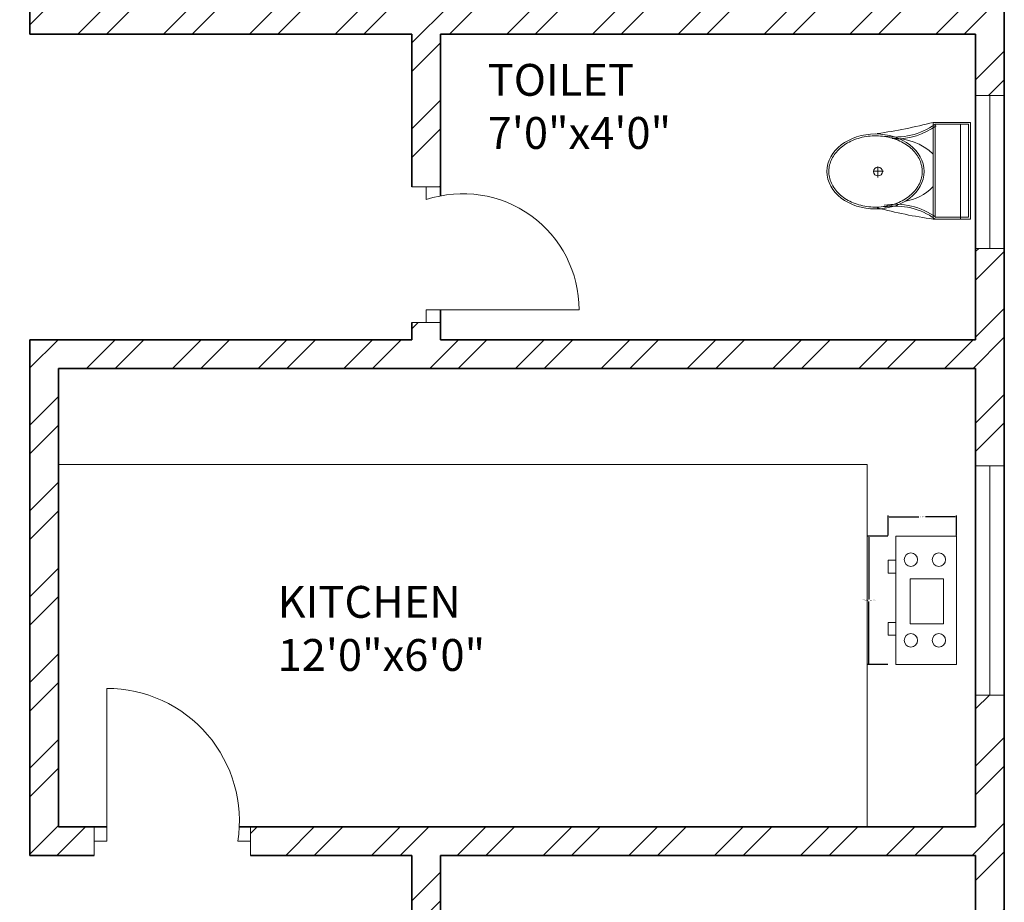
# Model space of a CAD drawing. Units: inches. Extents: x 1962 to 2771, y 1245 to 2660.
# Tile 20 of 114: x 2506 to 2661, y 1692 to 1831. Entities that reach past the tile are written whole.
import ezdxf

# ---------------------------------------------------------------- set-up
doc = ezdxf.new("R2010")
doc.units = ezdxf.units.IN
for name, color, linetype, lineweight in [('A-ANNO-DIMS', 2, 'Continuous', 18), ('A-AREA-IDEN', 7, 'Continuous', 18), ('A-DOOR', 3, 'Continuous', 18), ('A-EQPM', 8, 'Continuous', 18), ('A-FLOR-CASE', 8, 'Continuous', 18), ('A-FLOR-FIXT', 8, 'Continuous', 18), ('A-GLAZ', 4, 'Continuous', 18), ('A-WALL', 7, 'Continuous', 35), ('A-WALL-PATT', 252, 'Continuous', 13)]:
    doc.layers.add(name, color=color, linetype=linetype, lineweight=lineweight)
doc.styles.get("Standard").update_dxf_attribs({"font": 'arial.ttf'})
doc.dimstyles.get("Standard").update_dxf_attribs({"dimtxt": 0.18, "dimasz": 0.18, "dimexe": 0.18, "dimexo": 0.0625, "dimgap": 0.09, "dimtad": 0, "dimtih": 1, "dimtoh": 1, "dimdec": 4, "dimzin": 0, "dimdsep": 46, "dimtxsty": 'Standard', "dimcen": 0.09, "dimadec": 0, "dimazin": 0, "dimtfac": 1, "dimtdec": 4, "dimtofl": 0, "dimtmove": 0, "dimatfit": 3, "dimfxl": 1, "dimtolj": 1, "dimtzin": 0, "dimarcsym": 0})

# ---------------------------------------------------------------- blocks, each defined once
blk = doc.blocks.new('A$C31115884')
for p, q in [((283.1, 497.7), (223.4, 497.7)), ((257.5, 466.4), (257.5, 523.2)), ((0, 200), (0, 0)), ((520, 200), (0, 200)), ((10, 190), (10, 10)), ((510, 190), (10, 190)), ((510, 10), (510, 190)), ((520, 0), (520, 200)), ((510, 54.5), (0, 54.5)), ((10, 10), (510, 10)), ((0, 0), (520, 0))]:
    blk.add_line(p, q)
blk.add_circle((255.6, 496.4), 23.6)
for centre, radius, start, end in [((2777.7, -204.6), 2807, 165.4549, 171.7133), ((3237, 905), 2807, 188.2867, 194.5451), ((-294.5, 403.3), 364.7, 324.2091, 9.3499), ((-294.5, 403.3), 374.7, 324.2091, 9.3499), ((805.8, 403.3), 364.7, 170.6501, 215.7909), ((139.5, 406.2), 293.5, 315.8436, 2.6563), ((805.8, 403.3), 374.7, 179.2036, 215.7909), ((383.6, 406.2), 293.5, 190.2774, 224.1564)]:
    blk.add_arc(centre, radius, start, end)
blk.add_ellipse((256.2, 509.9), major_axis=(0, -260.7), ratio=0.772727)
blk.add_open_spline([(256.2, 259.2), (263.1, 259.2), (270, 259.7), (287.8, 262.3), (298.7, 265.1), (319.9, 273.1), (330.2, 278.4), (350.1, 291.1), (359.7, 298.7), (377.7, 315.9), (386.2, 325.5), (401.7, 346.6), (408.8, 358.1), (421.3, 382.5), (426.8, 395.5), (435.9, 422.4), (439.5, 436.4), (444.8, 465.1), (446.5, 479.7), (447.9, 509.2), (447.6, 524), (445, 553.3), (442.7, 567.8), (436.3, 596), (432.1, 609.7), (421.9, 636), (416, 648.6), (402.5, 672.1), (395, 683), (378.6, 703), (369.8, 712.1), (351.1, 728), (341.3, 734.8), (320.9, 746.2), (310.4, 750.7), (288.9, 757.3), (278, 759.4), (256, 761), (245, 760.6), (223.1, 757.2), (212.3, 754.3), (191.1, 746.1), (180.8, 740.7), (160.9, 727.8), (151.4, 720.1), (133.5, 702.7), (125.1, 693), (109.6, 671.7), (102.6, 660.2), (90.2, 635.7), (84.9, 622.7), (76, 595.6), (72.4, 581.6), (67.2, 552.9), (65.6, 538.2), (64.4, 508.8), (64.8, 494), (67.5, 464.7), (69.9, 450.2), (76.6, 422), (80.8, 408.3), (91.1, 382.2), (97.2, 369.7), (110.8, 346.3), (118.4, 335.4), (134.8, 315.6), (143.7, 306.7), (162.4, 290.9), (172.3, 284.2), (192.8, 273), (203.3, 268.6), (224.8, 262.2), (235.8, 260.2), (249.9, 259.3), (253, 259.2), (256.2, 259.2)], degree=3, knots=[0, 0, 0, 0, 0.110105, 0.110105, 0.285049, 0.285049, 0.459994, 0.459994, 0.634938, 0.634938, 0.809882, 0.809882, 0.984827, 0.984827, 1.159771, 1.159771, 1.334715, 1.334715, 1.50966, 1.50966, 1.684604, 1.684604, 1.859549, 1.859549, 2.034493, 2.034493, 2.209437, 2.209437, 2.384382, 2.384382, 2.559326, 2.559326, 2.73427, 2.73427, 2.909215, 2.909215, 3.084159, 3.084159, 3.259103, 3.259103, 3.434048, 3.434048, 3.608992, 3.608992, 3.783936, 3.783936, 3.958881, 3.958881, 4.133825, 4.133825, 4.30877, 4.30877, 4.483714, 4.483714, 4.658658, 4.658658, 4.833603, 4.833603, 5.008547, 5.008547, 5.183491, 5.183491, 5.358436, 5.358436, 5.53338, 5.53338, 5.708324, 5.708324, 5.883269, 5.883269, 6.058213, 6.058213, 6.233158, 6.233158, 6.283185, 6.283185, 6.283185, 6.283185])
blk = doc.blocks.new('COOKTOP-4-BURNER')
for points in [[(0, 20.18), (9.48, 20.18), (9.48, 0), (0, 0)], [(9.48, 15.59), (10.71, 15.59), (10.71, 13.59), (9.48, 13.59)], [(2, 13.79), (7.26, 13.79), (7.26, 6.73), (2, 6.73)], [(9.48, 5.81), (10.71, 5.81), (10.71, 3.8), (9.48, 3.8)]]:
    blk.add_lwpolyline(points, close=True)
for centre in [(2.74, 16.38), (7.14, 16.38), (2.74, 3.71), (7.14, 3.71)]:
    blk.add_circle(centre, 1.05)
blk = doc.blocks.new('WIN-24IN-A')
for p, q in [((0, 24), (4.5, 24)), ((4.5, 24), (2.25, 24)), ((2.25, 24), (2.25, 0)), ((2.25, 0), (0, 0)), ((0, 0), (4.5, 0))]:
    blk.add_line(p, q)
blk = doc.blocks.new('WIN-36IN-B')
for p, q in [((0, 36), (4.5, 36)), ((4.5, 36), (2.25, 36)), ((2.25, 36), (2.25, 0)), ((2.25, 0), (0, 0)), ((0, 0), (4.5, 0))]:
    blk.add_line(p, q)
blk = doc.blocks.new('*D30')
at = {"layer": 'A-ANNO-DIMS', "color": 0, "lineweight": -2, "transparency": 16777216}
for p, q in [((2642.51, 1749.52), (2639.37, 1749.52)), ((2639.55, 1749.34), (2639.55, 1739.61)), ((2639.55, 1729.52), (2639.55, 1739.25)), ((2642.51, 1729.34), (2639.37, 1729.34))]:
    blk.add_line(p, q, dxfattribs=at)
at = {"layer": 'A-ANNO-DIMS', "color": 0, "transparency": 16777216}
for points in [[(2639.52, 1749.34), (2639.58, 1749.34), (2639.55, 1749.52)], [(2639.52, 1729.52), (2639.58, 1729.52), (2639.55, 1729.34)]]:
    blk.add_solid(points, dxfattribs=at)
at = {"layer": 'Defpoints', "color": 0, "transparency": 16777216}
for p in [(2642.57, 1749.52), (2639.55, 1729.34), (2642.57, 1729.34)]:
    blk.add_point(p, dxfattribs=at)
at = {"layer": 'A-ANNO-DIMS', "color": 0, "transparency": 16777216, "insert": (2639.55, 1739.43), "char_height": 0.18, "attachment_point": 5}
blk.add_mtext('\\A1;COOKTOP 20 TYP.', dxfattribs=at)
blk = doc.blocks.new('*D31')
at = {"layer": 'A-ANNO-DIMS', "color": 0, "lineweight": -2, "transparency": 16777216}
for p, q in [((2642.57, 1749.58), (2642.57, 1752.72)), ((2642.75, 1752.54), (2647.41, 1752.54)), ((2653.1, 1752.54), (2648.45, 1752.54)), ((2653.28, 1749.58), (2653.28, 1752.72))]:
    blk.add_line(p, q, dxfattribs=at)
at = {"layer": 'A-ANNO-DIMS', "color": 0, "transparency": 16777216}
for points in [[(2642.75, 1752.57), (2642.75, 1752.51), (2642.57, 1752.54)], [(2653.1, 1752.57), (2653.1, 1752.51), (2653.28, 1752.54)]]:
    blk.add_solid(points, dxfattribs=at)
at = {"layer": 'Defpoints', "color": 0, "transparency": 16777216}
for p in [(2642.57, 1752.54), (2642.57, 1749.52), (2653.28, 1749.52)]:
    blk.add_point(p, dxfattribs=at)
at = {"layer": 'A-ANNO-DIMS', "color": 0, "transparency": 16777216, "insert": (2647.93, 1752.54), "char_height": 0.18, "attachment_point": 5}
blk.add_mtext('\\A1;11 TYP.', dxfattribs=at)

msp = doc.modelspace()

# ---------------------------------------------------------------- hatches: boundary and pattern name
at = {"layer": 'A-WALL-PATT'}
h = msp.add_hatch(dxfattribs=at)
h.set_pattern_fill('ANSI32', color=256)
h.paths.add_polyline_path([(2090.8074, 2467.3437), (2141.6481, 2467.3437), (2141.6481, 2469.5937), (2141.6481, 2471.8437), (2086.3074, 2471.8437), (2086.3074, 2422.5333), (2090.8074, 2422.5333)])
h.paths.add_polyline_path([(2282.7664, 2471.8437), (2204.8982, 2471.8437), (2204.8982, 2467.3437), (2234.8074, 2467.3437), (2234.8074, 2311.3437), (2228.7492, 2311.3437), (2228.7492, 2306.8437), (2234.8074, 2306.8437), (2331.9227, 2306.8437), (2331.9227, 2309.0937), (2331.9227, 2311.3437), (2239.3074, 2311.3437), (2239.3074, 2467.3437), (2282.7664, 2467.3437), (2282.7664, 2469.5937)])
h.paths.add_polyline_path([(2471.4531, 2519.8437), (2552.011, 2519.8437), (2564.3996, 2519.8437), (2564.3996, 2511.1389), (2568.8996, 2511.1389), (2568.8996, 2524.3437), (2466.9531, 2524.3437), (2466.9531, 2471.8437), (2450.0749, 2471.8437), (2446.4672, 2471.8437), (2446.4672, 2467.3437), (2450.0749, 2467.3437), (2475.9988, 2467.3437), (2475.9988, 2469.5937), (2475.9988, 2471.8437), (2471.4531, 2471.8437)])
h.paths.add_polyline_path([(2575.2231, 2469.5937), (2575.2231, 2471.8437), (2568.8996, 2471.8437), (2568.8996, 2487.1389), (2564.3996, 2487.1389), (2564.3996, 2471.8437), (2556.511, 2471.8437), (2499.2904, 2471.8437), (2499.2904, 2467.3437), (2507.8074, 2467.3437), (2507.8074, 2311.3437), (2414.863, 2311.3437), (2414.863, 2306.8437), (2512.3074, 2306.8437), (2517.0114, 2306.8437), (2517.0114, 2309.0937), (2517.0114, 2311.3437), (2512.3074, 2311.3437), (2512.3074, 2467.3437), (2575.2231, 2467.3437)])
h.paths.add_polyline_path([(2660.8074, 2471.8437), (2600.9602, 2471.8437), (2600.9602, 2467.3437), (2656.3074, 2467.3437), (2656.3074, 2432.5704), (2660.8074, 2432.5704)])
h.paths.add_polyline_path([(2660.8074, 2372.5704), (2656.3074, 2372.5704), (2656.3074, 2311.3437), (2600.276, 2311.3437), (2600.276, 2309.0937), (2600.276, 2306.8437), (2656.3074, 2306.8437), (2656.3074, 2296.2593), (2660.8074, 2296.2593)])
h.paths.add_polyline_path([(2572.3074, 2306.8437), (2577.1385, 2306.8437), (2577.1385, 2311.3437), (2551.082, 2311.3437), (2551.082, 2306.8437), (2567.8074, 2306.8437), (2567.8074, 2258.8437), (2540.0574, 2258.8437), (2540.0574, 2256.5937), (2540.0574, 2254.3437), (2567.8074, 2254.3437), (2656.3074, 2254.3437), (2656.3074, 2236.9085), (2660.8074, 2236.9085), (2660.8074, 2272.2593), (2656.3074, 2272.2593), (2656.3074, 2258.8437), (2572.3074, 2258.8437)])
h.paths.add_polyline_path([(2512.3074, 2254.3437), (2518.8716, 2254.3437), (2518.8716, 2256.5937), (2518.8716, 2258.8437), (2507.8074, 2258.8437), (2507.8074, 2177.8437), (2567.8074, 2177.8437), (2567.8074, 2172.9628), (2572.3074, 2172.9628), (2572.3074, 2177.8437), (2656.3074, 2177.8437), (2656.3074, 2166.4846), (2660.8074, 2166.4846), (2660.8074, 2200.9085), (2656.3074, 2200.9085), (2656.3074, 2182.3437), (2512.3074, 2182.3437)])
h.paths.add_polyline_path([(2656.3074, 2129.8437), (2572.3074, 2129.8437), (2572.3074, 2150.3044), (2570.0574, 2150.3044), (2567.8074, 2150.3044), (2567.8074, 2129.8437), (2507.8074, 2129.8437), (2507.8074, 2116.3027), (2510.0574, 2116.3027), (2512.3074, 2116.3027), (2512.3074, 2125.3437), (2567.8074, 2125.3437), (2572.3074, 2125.3437), (2656.3074, 2125.3437)])
h.paths.add_polyline_path([(2090.8074, 2362.5333), (2086.3074, 2362.5333), (2086.3074, 2298.6242), (2090.8074, 2298.6242), (2090.8074, 2306.8437), (2174.8074, 2306.8437), (2174.8074, 2286.4178), (2179.3074, 2286.4178), (2179.3074, 2306.8437), (2192.8641, 2306.8437), (2192.8641, 2309.0937), (2192.8641, 2311.3437), (2090.8074, 2311.3437)])
h.paths.add_polyline_path([(2209.156, 2258.8437), (2179.3074, 2258.8437), (2179.3074, 2263.2236), (2177.0574, 2263.2236), (2174.8074, 2263.2236), (2174.8074, 2258.8437), (2090.8074, 2258.8437), (2090.8074, 2274.6242), (2086.3074, 2274.6242), (2086.3074, 2238.2967), (2088.5574, 2238.2967), (2090.8074, 2238.2967), (2090.8074, 2254.3437), (2209.156, 2254.3437)])
h.paths.add_polyline_path([(2090.8074, 2177.8437), (2234.8074, 2177.8437), (2234.8074, 2173.1428), (2239.3074, 2173.1428), (2239.3074, 2258.8437), (2230.8442, 2258.8437), (2230.8442, 2256.5937), (2230.8442, 2254.3437), (2234.8074, 2254.3437), (2234.8074, 2182.3437), (2090.8074, 2182.3437), (2090.8074, 2202.2967), (2086.3074, 2202.2967), (2086.3074, 2140.0389), (2090.8074, 2140.0389)])
h.paths.add_polyline_path([(2090.8074, 2080.0389), (2086.3074, 2080.0389), (2086.3074, 2033.8437), (2090.8074, 2033.8437)], flags=17)
h.paths.add_polyline_path([(2244.9405, 2033.8437), (2239.3074, 2033.8437), (2239.3074, 2142.0665), (2237.2592, 2142.0665), (2234.8074, 2142.0665), (2234.8074, 2033.8437), (2090.8074, 2033.8437), (2076.5204, 2033.8437), (2072.0204, 2033.8437), (2072.0204, 2000.4493), (2076.5204, 2000.4493), (2076.5204, 2029.3437), (2090.8074, 2029.3437), (2244.9405, 2029.3437), (2244.9405, 2031.5937)])
h.paths.add_polyline_path([(2234.8074, 1933.3437), (2076.5204, 1933.3437), (2076.5204, 1952.4493), (2074.2704, 1952.4493), (2072.0204, 1952.4493), (2072.0204, 1933.3437), (2072.0204, 1928.8437), (2234.8074, 1928.8437)])
h.paths.add_polyline_path([(2090.8074, 1928.8437), (2086.3074, 1928.8437), (2086.3074, 1906.5013), (2090.8074, 1906.5013)])
h.paths.add_polyline_path([(2090.8074, 1846.5013), (2086.3074, 1846.5013), (2086.3074, 1769.9917), (2088.5574, 1769.9917), (2090.8074, 1769.9917), (2090.8074, 1780.3437), (2234.8074, 1780.3437), (2234.8074, 1708.3437), (2230.3764, 1708.3437), (2230.3764, 1703.8437), (2239.3074, 1703.8437), (2239.3074, 1792.6669), (2237.0574, 1792.6669), (2234.8074, 1792.6669), (2234.8074, 1784.8437), (2090.8074, 1784.8437)])
h.paths.add_polyline_path([(2239.3074, 1928.8437), (2244.9405, 1928.8437), (2244.9405, 1931.0937), (2244.9405, 1933.3437), (2234.8074, 1933.3437), (2234.8074, 1928.8437), (2234.8074, 1825.5949), (2239.3074, 1825.5949)])
h.paths.add_polyline_path([(2148.0425, 1649.0937), (2148.0425, 1651.3437), (2090.8074, 1651.3437), (2090.8074, 1646.8437), (2148.0425, 1646.8437)], flags=0)
h.paths.add_polyline_path([(2207.5601, 1708.3437), (2090.8074, 1708.3437), (2090.8074, 1703.8437), (2174.8074, 1703.8437), (2174.8074, 1651.3437), (2170.4457, 1651.3437), (2170.4457, 1646.8437), (2195.9924, 1646.8437), (2195.9924, 1649.0937), (2195.9924, 1651.3437), (2179.3074, 1651.3437), (2179.3074, 1703.8437), (2207.5601, 1703.8437), (2207.5601, 1706.0937)])
h.paths.add_polyline_path([(2090.8074, 1733.9917), (2086.3074, 1733.9917), (2086.3074, 1696.1032), (2088.5574, 1696.1032), (2090.8074, 1696.1032)])
h.paths.add_polyline_path([(2090.8074, 1672.1032), (2086.3074, 1672.1032), (2086.3074, 1600.3335), (2090.8074, 1600.3335)])
h.paths.add_polyline_path([(2090.8074, 1540.3335), (2086.3074, 1540.3335), (2086.3074, 1486.3437), (2139.6766, 1486.3437), (2139.6766, 1490.8437), (2090.8074, 1490.8437)])
h.paths.add_polyline_path([(2302.3876, 1490.8437), (2239.3074, 1490.8437), (2239.3074, 1646.8437), (2335.9994, 1646.8437), (2335.9994, 1651.3437), (2229.884, 1651.3437), (2229.884, 1646.8437), (2234.8074, 1646.8437), (2234.8074, 1490.8437), (2202.7103, 1490.8437), (2202.7103, 1488.5937), (2202.7103, 1486.3437), (2275.0699, 1486.3437), (2275.0699, 1475.772), (2279.5699, 1475.772), (2279.5699, 1486.3437), (2302.3876, 1486.3437)])
h.paths.add_polyline_path([(2279.5699, 1451.772), (2275.0699, 1451.772), (2275.0699, 1438.3437), (2174.8074, 1438.3437), (2174.8074, 1486.3437), (2179.7922, 1486.3437), (2179.7922, 1490.8437), (2163.3585, 1490.8437), (2163.3585, 1488.5937), (2163.3585, 1486.3437), (2170.3074, 1486.3437), (2170.3074, 1433.8437), (2279.5699, 1433.8437)])
h.paths.add_polyline_path([(2427.2363, 1490.8437), (2375.8074, 1490.8437), (2375.8074, 1646.8437), (2381.6401, 1646.8437), (2381.6401, 1651.3437), (2365.887, 1651.3437), (2365.887, 1649.0937), (2365.887, 1646.8437), (2371.3074, 1646.8437), (2371.3074, 1490.8437), (2327.5627, 1490.8437), (2327.5627, 1488.5937), (2327.5627, 1486.3437), (2371.3074, 1486.3437), (2371.3074, 1433.8437), (2375.8074, 1433.8437), (2375.8074, 1486.3437), (2427.2363, 1486.3437)])
h.paths.add_polyline_path([(2512.3074, 1646.8437), (2519.4351, 1646.8437), (2519.4351, 1649.0937), (2519.4351, 1651.3437), (2507.8074, 1651.3437), (2416.0063, 1651.3437), (2416.0063, 1649.0937), (2416.0063, 1646.8437), (2507.8074, 1646.8437), (2507.8074, 1490.8437), (2497.0532, 1490.8437), (2497.0532, 1488.5937), (2497.0532, 1486.3437), (2574.9344, 1486.3437), (2574.9344, 1476.0181), (2579.4344, 1476.0181), (2579.4344, 1486.3437), (2584.4872, 1486.3437), (2584.3074, 1490.8437), (2512.3074, 1490.8437)])
h.paths.add_polyline_path([(2470.5091, 1486.3437), (2473.9767, 1486.3437), (2473.9767, 1490.8437), (2449.6605, 1490.8437), (2449.6605, 1488.5937), (2449.6605, 1486.3437), (2466.0091, 1486.3437), (2466.0091, 1433.8437), (2470.5091, 1433.8437), (2579.4344, 1433.8437), (2579.4344, 1452.0181), (2574.9344, 1452.0181), (2574.9344, 1438.3437), (2554.5091, 1438.3437), (2470.5091, 1438.3437)])
h.paths.add_polyline_path([(2656.3074, 1490.8437), (2611.86, 1490.8437), (2611.86, 1486.3437), (2656.3074, 1486.3437)])
h.paths.add_polyline_path([(2660.8074, 1532.7007), (2658.5574, 1532.7007), (2656.3074, 1532.7007), (2656.3074, 1486.3437), (2660.8074, 1486.3437)])
h.paths.add_polyline_path([(2660.8074, 1664.9663), (2656.3074, 1664.9663), (2656.3074, 1651.3437), (2602.2313, 1651.3437), (2602.2313, 1646.8437), (2656.3074, 1646.8437), (2656.3074, 1592.7007), (2660.8074, 1592.7007)])
h.paths.add_polyline_path([(2660.8074, 1724.5221), (2656.3074, 1724.5221), (2656.3074, 1703.8437), (2542.4725, 1703.8437), (2542.4725, 1699.3437), (2567.8074, 1699.3437), (2567.8074, 1651.3437), (2552.7766, 1651.3437), (2552.7766, 1649.0937), (2552.7766, 1646.8437), (2577.2878, 1646.8437), (2577.2878, 1649.0937), (2577.2878, 1651.3437), (2572.3074, 1651.3437), (2572.3074, 1699.3437), (2656.3074, 1699.3437), (2656.3074, 1688.9663), (2660.8074, 1688.9663)])
h.paths.add_polyline_path([(2660.8074, 1880.6524), (2656.3074, 1880.6524), (2656.3074, 1832.8437), (2512.3074, 1832.8437), (2512.3074, 1837.8959), (2507.8074, 1837.8959), (2507.8074, 1828.3437), (2567.8074, 1828.3437), (2567.8074, 1804.3437), (2572.3074, 1804.3437), (2572.3074, 1828.3437), (2656.3074, 1828.3437), (2656.3074, 1818.6778), (2660.8074, 1818.6778)])
h.paths.add_polyline_path([(2660.8074, 1794.6778), (2656.3074, 1794.6778), (2656.3074, 1780.3437), (2572.3074, 1780.3437), (2572.3074, 1783.0303), (2570.0574, 1783.0303), (2567.8074, 1783.0303), (2567.8074, 1780.3437), (2507.8074, 1780.3437), (2507.8074, 1699.3437), (2517.8858, 1699.3437), (2517.8858, 1701.5937), (2517.8858, 1703.8437), (2512.3074, 1703.8437), (2512.3074, 1775.8437), (2656.3074, 1775.8437), (2656.3074, 1760.5221), (2660.8074, 1760.5221)])
h.paths.add_polyline_path([(2660.8074, 1981.3437), (2660.8074, 2020.2808), (2658.5574, 2020.2808), (2656.3074, 2020.2808), (2656.3074, 1981.3437), (2512.3074, 1981.3437), (2512.3074, 2086.6996), (2507.8074, 2086.6996), (2507.8074, 1981.3437), (2375.8074, 1981.3437), (2375.8074, 1986.8505), (2373.5574, 1986.8505), (2371.3074, 1986.8505), (2371.3074, 1973.2607), (2375.8074, 1973.2607), (2375.8074, 1976.8437), (2507.8074, 1976.8437), (2507.8074, 1865.4281), (2510.0574, 1865.4281), (2512.3074, 1865.4281), (2512.3074, 1976.8437), (2660.8074, 1976.8437)])
h.paths.add_polyline_path([(2375.8074, 1940.297), (2373.5574, 1940.297), (2371.3074, 1940.297), (2371.3074, 1933.3437), (2278.4434, 1933.3437), (2278.4434, 1928.8437), (2371.3074, 1928.8437), (2371.3074, 1651.3437), (2375.8074, 1651.3437)])
h.paths.add_polyline_path([(2660.8074, 1976.8437), (2656.3074, 1976.8437), (2656.3074, 1940.6524), (2660.8074, 1940.6524)], flags=17)
h.paths.add_polyline_path([(2660.8074, 2142.4846), (2656.3074, 2142.4846), (2656.3074, 2080.2808), (2660.8074, 2080.2808)])
h.paths.add_polyline_path([(2381.4189, 2311.3437), (2375.8074, 2311.3437), (2375.8074, 2467.3437), (2424.7242, 2467.3437), (2424.7242, 2469.5937), (2424.7242, 2471.8437), (2375.8074, 2471.8437), (2375.8074, 2524.3437), (2371.3074, 2524.3437), (2371.3074, 2471.8437), (2307.2097, 2471.8437), (2307.2097, 2467.3437), (2371.3074, 2467.3437), (2371.3074, 2311.3437), (2366.8901, 2311.3437), (2366.8901, 2306.8437), (2371.3074, 2306.8437), (2371.3074, 2033.8437), (2279.6589, 2033.8437), (2279.6589, 2029.3437), (2371.3074, 2029.3437), (2371.3074, 2014.2598), (2375.8074, 2014.2598), (2375.8074, 2306.8437), (2381.4189, 2306.8437)])
h.paths.add_polyline_path([(2263.3074, 2524.3437), (2170.3074, 2524.3437), (2170.3074, 2519.8437), (2170.3074, 2471.8437), (2165.0312, 2471.8437), (2165.0312, 2467.3437), (2179.6721, 2467.3437), (2179.6721, 2469.5161), (2179.6721, 2471.8437), (2174.8074, 2471.8437), (2174.8074, 2519.8437), (2258.8074, 2519.8437), (2258.8074, 2511.6436), (2263.3074, 2511.6436)])
h.paths.add_polyline_path([(2245.0232, 1361.4123), (2492.9468, 1361.4123), (2492.9468, 1398.505), (2245.0232, 1398.505)], flags=9)
h.paths.add_polyline_path([(2388.1434, 2086.6936), (2425.0704, 2086.6936), (2425.0704, 2105.3509), (2388.1434, 2105.3509)], flags=9)
h.paths.add_polyline_path([(2404.922, 2242.6744), (2445.7337, 2242.6744), (2445.7337, 2261.3318), (2404.922, 2261.3318)], flags=9)
h.paths.add_polyline_path([(2269.4107, 2156.7935), (2306.3378, 2156.7935), (2306.3378, 2175.4508), (2269.4107, 2175.4508)], flags=9)
h.paths.add_polyline_path([(2269.3277, 2233.4343), (2306.2547, 2233.4343), (2306.2547, 2252.0917), (2269.3277, 2252.0917)], flags=9)
h.paths.add_polyline_path([(2431.6052, 2320.6922), (2470.4456, 2320.6922), (2470.4456, 2339.3495), (2431.6052, 2339.3495)], flags=25)
h.paths.add_polyline_path([(2249.6902, 2315.7608), (2288.5306, 2315.7608), (2288.5306, 2334.4182), (2249.6902, 2334.4182)], flags=25)
h.paths.add_polyline_path([(2096.9301, 2314.3181), (2135.7704, 2314.3181), (2135.7704, 2332.9755), (2096.9301, 2332.9755)], flags=25)
h.paths.add_polyline_path([(2134.3475, 2285.7089), (2161.4655, 2285.7089), (2161.4655, 2304.3662), (2134.3475, 2304.3662)], flags=9)
h.paths.add_polyline_path([(2126.5155, 2209.4076), (2159.9227, 2209.4076), (2159.9227, 2228.065), (2126.5155, 2228.065)], flags=25)
h.paths.add_polyline_path([(2110.5753, 2141.5299), (2149.4157, 2141.5299), (2149.4157, 2160.1872), (2110.5753, 2160.1872)], flags=25)
h.paths.add_polyline_path([(2249.8618, 1968.3317), (2286.3966, 1968.3317), (2286.3966, 1986.989), (2249.8618, 1986.989)], flags=9)
h.paths.add_polyline_path([(2395.9507, 1777.0051), (2436.7624, 1777.0051), (2436.7624, 1795.6625), (2395.9507, 1795.6625)], flags=9)
h.paths.add_polyline_path([(2398.5259, 1888.5651), (2435.0062, 1888.5651), (2435.0062, 1907.2224), (2398.5259, 1907.2224)], flags=25)
h.paths.add_polyline_path([(2259.3506, 1728.3559), (2296.2776, 1728.3559), (2296.2776, 1747.0132), (2259.3506, 1747.0132)], flags=9)
h.paths.add_polyline_path([(2271.3698, 1845.268), (2308.2968, 1845.268), (2308.2968, 1863.9253), (2271.3698, 1863.9253)], flags=9)
h.paths.add_polyline_path([(2120.9355, 1786.3027), (2159.7759, 1786.3027), (2159.7759, 1804.9601), (2120.9355, 1804.9601)], flags=25)
h.paths.add_polyline_path([(2121.3164, 1732.1043), (2154.7236, 1732.1043), (2154.7236, 1750.7616), (2121.3164, 1750.7616)], flags=25)
h.paths.add_polyline_path([(2118.3706, 1678.8997), (2147.5282, 1678.8997), (2147.5282, 1697.557), (2118.3706, 1697.557)], flags=25)
h.paths.add_polyline_path([(2385.9227, 1493.557), (2424.763, 1493.557), (2424.763, 1512.2143), (2385.9227, 1512.2143)], flags=25)
h.paths.add_polyline_path([(2248.7058, 1500.0256), (2287.5462, 1500.0256), (2287.5462, 1518.6829), (2248.7058, 1518.6829)], flags=25)
h.paths.add_polyline_path([(2104.1669, 1617.3771), (2143.0073, 1617.3771), (2143.0073, 1636.0344), (2104.1669, 1636.0344)], flags=9)
h.paths.add_polyline_path([(2096.0714, 1447.8824), (2137.3845, 1447.8824), (2137.3845, 1458.1859), (2096.0714, 1458.1859)], flags=9)
h.paths.add_polyline_path([(2180.6114, 1440.325), (2209.7689, 1440.325), (2209.7689, 1458.9823), (2180.6114, 1458.9823)], flags=25)
h.paths.add_polyline_path([(2316.1698, 1447.9637), (2357.4829, 1447.9637), (2357.4829, 1458.2673), (2316.1698, 1458.2673)], flags=9)
h.paths.add_polyline_path([(2397.6187, 1447.9637), (2438.9318, 1447.9637), (2438.9318, 1458.2673), (2397.6187, 1458.2673)], flags=9)
h.paths.add_polyline_path([(2473.0778, 1439.5953), (2502.2354, 1439.5953), (2502.2354, 1458.2527), (2473.0778, 1458.2527)], flags=25)
h.paths.add_polyline_path([(2589.7027, 1447.8819), (2631.0158, 1447.8819), (2631.0158, 1458.1855), (2589.7027, 1458.1855)], flags=9)
h.paths.add_polyline_path([(2522.4009, 1497.5285), (2561.2413, 1497.5285), (2561.2413, 1516.1859), (2522.4009, 1516.1859)], flags=25)
h.paths.add_polyline_path([(2579.6565, 1671.3482), (2608.8141, 1671.3482), (2608.8141, 1690.0056), (2579.6565, 1690.0056)], flags=25)
h.paths.add_polyline_path([(2544.7038, 1725.5064), (2578.1111, 1725.5064), (2578.1111, 1744.1637), (2544.7038, 1744.1637)], flags=25)
h.paths.add_polyline_path([(2578.1191, 1807.472), (2607.2766, 1807.472), (2607.2766, 1826.1293), (2578.1191, 1826.1293)], flags=25)
h.paths.add_polyline_path([(2595.0614, 1835.1839), (2633.9018, 1835.1839), (2633.9018, 1853.8413), (2595.0614, 1853.8413)], flags=25)
h.paths.add_polyline_path([(2567.0097, 2097.7035), (2605.8501, 2097.7035), (2605.8501, 2116.3609), (2567.0097, 2116.3609)], flags=9)
h.paths.add_polyline_path([(2586.644, 2134.6454), (2615.8015, 2134.6454), (2615.8015, 2153.3027), (2586.644, 2153.3027)], flags=9)
h.paths.add_polyline_path([(2544.6185, 2212.6783), (2578.0258, 2212.6783), (2578.0258, 2231.3356), (2544.6185, 2231.3356)], flags=25)
h.paths.add_polyline_path([(2577.0273, 2256.9023), (2606.1849, 2256.9023), (2606.1849, 2275.5597), (2577.0273, 2275.5597)], flags=24)
h.paths.add_polyline_path([(2605.2683, 2315.2821), (2644.1087, 2315.2821), (2644.1087, 2333.9395), (2605.2683, 2333.9395)], flags=25)
h.paths.add_polyline_path([(2583.1244, 2496.1815), (2624.4375, 2496.1815), (2624.4375, 2506.4851), (2583.1244, 2506.4851)], flags=9)
h.paths.add_polyline_path([(2474.761, 2497.0823), (2503.9185, 2497.0823), (2503.9185, 2515.7397), (2474.761, 2515.7397)], flags=25)
h.paths.add_polyline_path([(2387.5787, 2494.2563), (2428.902, 2494.2563), (2428.902, 2504.5598), (2387.5787, 2504.5598)], flags=9)
h.paths.add_polyline_path([(2300.1657, 2500.1564), (2341.4788, 2500.1564), (2341.4788, 2510.46), (2300.1657, 2510.46)], flags=25)
h.paths.add_polyline_path([(2176.8589, 2497.5843), (2206.0165, 2497.5843), (2206.0165, 2516.2416), (2176.8589, 2516.2416)], flags=25)
h.paths.add_polyline_path([(2097.4668, 2494.9762), (2138.7799, 2494.9762), (2138.7799, 2505.2798), (2097.4668, 2505.2798)], flags=9)

# ---------------------------------------------------------------- linework, layer by layer
at = {"layer": 'A-DOOR'}
for p, q in [((2567.8074, 1804.3437), (2572.3074, 1804.3437)), ((2572.3074, 1804.3437), (2570.0574, 1804.3437)), ((2570.0574, 1804.3437), (2570.0574, 1802.3437)), ((2570.0574, 1783.0303), (2570.0574, 1785.0303)), ((2570.0574, 1785.0303), (2594.0574, 1785.0303)), ((2567.8074, 1783.0303), (2572.3074, 1783.0303)), ((2572.3074, 1783.0303), (2570.0574, 1783.0303)), ((2519.8858, 1701.5937), (2519.8858, 1725.5937)), ((2517.8858, 1703.8437), (2517.8858, 1699.3437)), ((2542.4725, 1703.8437), (2542.4725, 1699.3437)), ((2517.8858, 1699.3437), (2517.8858, 1701.5937)), ((2517.8858, 1701.5937), (2519.8858, 1701.5937)), ((2542.4725, 1701.5937), (2540.4725, 1701.5937)), ((2542.4725, 1699.3437), (2542.4725, 1701.5937))]:
    msp.add_line(p, q, dxfattribs=at)
for centre, radius, start, end in [((2575.8125, 1785.0303), 18.2449, 360, 108.387185), ((2519.8858, 1704.7643), 20.8294, 351.244592, 90)]:
    msp.add_arc(centre, radius, start, end, dxfattribs=at)
at = {"layer": 'A-FLOR-CASE'}
for p, q in [((2512.3074, 1760.7264), (2512.3074, 1760.7264)), ((2512.3074, 1760.7264), (2639.2816, 1760.7264)), ((2639.2816, 1760.7264), (2639.2816, 1703.8437))]:
    msp.add_line(p, q, dxfattribs=at)
at = {"layer": 'A-WALL'}
for p, q in [((2660.8074, 1976.8437), (2660.8074, 1486.3437)), ((2507.8074, 1837.8959), (2507.8074, 1828.3437)), ((2567.8074, 1828.3437), (2507.8074, 1828.3437)), ((2567.8074, 1804.3437), (2567.8074, 1828.3437)), ((2656.3074, 1828.3437), (2572.3074, 1828.3437)), ((2656.3074, 1828.3437), (2572.3074, 1828.3437)), ((2572.3074, 1828.3437), (2572.3074, 1802.9353)), ((2656.3074, 1828.3437), (2656.3074, 1780.3437)), ((2572.3074, 1785.0303), (2572.3074, 1780.3437)), ((2567.8074, 1780.3437), (2567.8074, 1783.0303)), ((2507.8074, 1780.3437), (2507.8074, 1699.3437)), ((2567.8074, 1780.3437), (2507.8074, 1780.3437)), ((2656.3074, 1780.3437), (2572.3074, 1780.3437)), ((2656.3074, 1775.8437), (2512.3074, 1775.8437)), ((2512.3074, 1775.8437), (2512.3074, 1703.8437)), ((2656.3074, 1775.8437), (2656.3074, 1703.8437)), ((2519.8858, 1703.8437), (2512.3074, 1703.8437)), ((2656.3074, 1703.8437), (2540.6949, 1703.8437)), ((2517.8858, 1699.3437), (2507.8074, 1699.3437)), ((2567.8074, 1699.3437), (2542.4725, 1699.3437)), ((2567.8074, 1651.3437), (2567.8074, 1699.3437)), ((2656.3074, 1699.3437), (2572.3074, 1699.3437)), ((2656.3074, 1699.3437), (2572.3074, 1699.3437)), ((2572.3074, 1699.3437), (2572.3074, 1651.3437)), ((2656.3074, 1699.3437), (2656.3074, 1651.3437))]:
    msp.add_line(p, q, dxfattribs=at)

# ---------------------------------------------------------------- block references
at = {"layer": 'A-EQPM', "rotation": 180}
msp.add_blockref('COOKTOP-4-BURNER', (2653.2809, 1749.5182), dxfattribs=at)
at = {"layer": 'A-FLOR-FIXT', "xscale": 0.0292470664339069, "yscale": 0.0292470664339069, "zscale": 0.0292470664339069, "rotation": 89.99999999999999}
msp.add_blockref('A$C31115884', (2655.5006, 1799.2674), dxfattribs=at)
at = {"layer": 'A-GLAZ'}
for name, p in [('WIN-24IN-A', (2656.3074, 1794.6778)), ('WIN-36IN-B', (2656.3074, 1724.5221))]:
    msp.add_blockref(name, p, dxfattribs=at)

# ---------------------------------------------------------------- texts
at = {"layer": 'A-AREA-IDEN', "char_height": 5, "attachment_point": 1}
for s, width, insert in [('TOILET\\P7\'0"x4\'0"', 86.563683, (2579.6999, 1823.6447)), ('KITCHEN\\P12\'0"x6\'0"', 153.438378, (2546.7144, 1741.6757))]:
    msp.add_mtext_dynamic_manual_height_columns(s, width=width, gutter_width=12.5, heights=[0], dxfattribs=dict(at, insert=insert))

# ---------------------------------------------------------------- dimensions: what is measured, and where the dimension line sits
at = {"layer": 'A-ANNO-DIMS'}
for base, p1, p2, angle, text, picture, middle in [((2642.5728, 1752.5448), (2653.2809, 1749.5182), (2642.5728, 1749.5182), 180, '<> TYP.', '*D31', (2647.9268, 1752.5448)), ((2639.5461, 1729.3405), (2642.5728, 1749.5182), (2642.5728, 1729.3405), 270, 'COOKTOP <> TYP.', '*D30', (2639.5461, 1739.4293))]:
    dim = msp.add_linear_dim(base=base, p1=p1, p2=p2, angle=angle, text=text, dimstyle='Standard', override={"dimdec": 0, "dimlfac": 1, "dimrnd": 0, "dimzin": 0, "dimdsep": 46, "dimlunit": 2}, dxfattribs=at)
    dim.commit()
    dim.dimension.update_dxf_attribs({"geometry": picture, "text_midpoint": middle})

doc.saveas('drawing.dxf')
